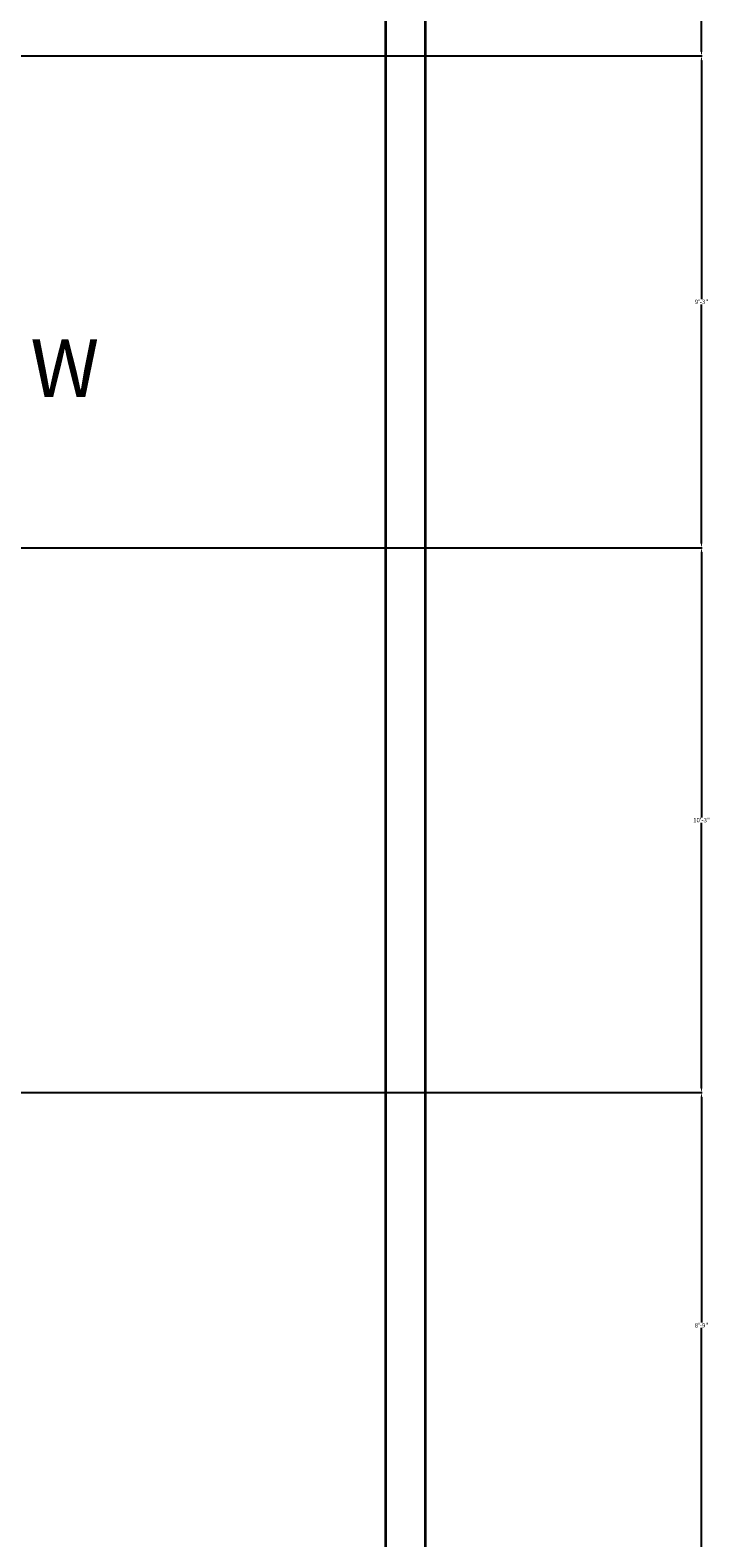
# Model space of a CAD drawing. Units: inches. Extents: x -364 to 705, y -52 to 1250.
# Tile 19 of 34: x 551 to 705, y 308 to 648. Entities that reach past the tile are written whole.
import ezdxf

# ---------------------------------------------------------------- set-up
doc = ezdxf.new("R2010")
doc.units = ezdxf.units.IN
doc.header["$MEASUREMENT"] = 0
for name, color, linetype, lineweight in [('A-ANNO-DIMS', 4, 'Continuous', 18), ('A-ANNO-IDEN', 1, 'Continuous', 18), ('C-WALL', 41, 'Continuous', 35)]:
    doc.layers.add(name, color=color, linetype=linetype, lineweight=lineweight)
doc.styles.get("Standard").update_dxf_attribs({"font": 'arial.ttf'})
doc.dimstyles.get("Standard").update_dxf_attribs({"dimtxt": 1, "dimasz": 1, "dimexe": 0.18, "dimexo": 0.0625, "dimgap": 0.09, "dimtad": 0, "dimtih": 1, "dimtoh": 1, "dimdec": 0, "dimzin": 0, "dimdsep": 46, "dimlunit": 3, "dimtxsty": 'Standard', "dimcen": 0.09, "dimadec": 0, "dimazin": 0, "dimtfac": 1, "dimtdec": 0, "dimtofl": 0, "dimtmove": 0, "dimatfit": 3, "dimfxl": 1, "dimtolj": 1, "dimtzin": 0, "dimarcsym": 0})

# ---------------------------------------------------------------- blocks, each defined once
blk = doc.blocks.new('*D79')
at = {"layer": 'A-ANNO-DIMS', "color": 0, "lineweight": -2, "transparency": 16777216}
for p, q in [((538.64, 408.11), (703.01, 408.11)), ((702.83, 407.11), (702.83, 356.22)), ((702.83, 304.11), (702.83, 355.01)), ((538.64, 303.11), (703.01, 303.11))]:
    blk.add_line(p, q, dxfattribs=at)
at = {"layer": 'A-ANNO-DIMS', "color": 0, "transparency": 16777216}
for points in [[(702.66, 407.11), (703, 407.11), (702.83, 408.11)], [(702.66, 304.11), (703, 304.11), (702.83, 303.11)]]:
    blk.add_solid(points, dxfattribs=at)
at = {"layer": 'Defpoints', "color": 0, "transparency": 16777216}
for p in [(538.58, 408.11), (702.83, 408.11), (538.58, 303.11)]:
    blk.add_point(p, dxfattribs=at)
at = {"layer": 'A-ANNO-DIMS', "color": 0, "transparency": 16777216, "insert": (702.83, 355.61), "char_height": 1, "attachment_point": 5}
blk.add_mtext('\\A1;8\'-9"', dxfattribs=at)
blk = doc.blocks.new('*D80')
at = {"layer": 'A-ANNO-DIMS', "color": 0, "lineweight": -2, "transparency": 16777216}
for p, q in [((538.64, 531.11), (703.01, 531.11)), ((702.83, 530.11), (702.83, 470.22)), ((702.83, 409.11), (702.83, 469.01)), ((538.64, 408.11), (703.01, 408.11))]:
    blk.add_line(p, q, dxfattribs=at)
at = {"layer": 'A-ANNO-DIMS', "color": 0, "transparency": 16777216}
for points in [[(702.66, 530.11), (703, 530.11), (702.83, 531.11)], [(702.66, 409.11), (703, 409.11), (702.83, 408.11)]]:
    blk.add_solid(points, dxfattribs=at)
at = {"layer": 'Defpoints', "color": 0, "transparency": 16777216}
for p in [(538.58, 531.11), (702.83, 531.11), (538.58, 408.11)]:
    blk.add_point(p, dxfattribs=at)
at = {"layer": 'A-ANNO-DIMS', "color": 0, "transparency": 16777216, "insert": (702.83, 469.61), "char_height": 1, "attachment_point": 5}
blk.add_mtext('\\A1;10\'-3"', dxfattribs=at)
blk = doc.blocks.new('*D81')
at = {"layer": 'A-ANNO-DIMS', "color": 0, "lineweight": -2, "transparency": 16777216}
for p, q in [((538.64, 642.11), (703.01, 642.11)), ((702.83, 641.11), (702.83, 587.22)), ((702.83, 532.11), (702.83, 586.01)), ((538.64, 531.11), (703.01, 531.11))]:
    blk.add_line(p, q, dxfattribs=at)
at = {"layer": 'A-ANNO-DIMS', "color": 0, "transparency": 16777216}
for points in [[(702.66, 641.11), (703, 641.11), (702.83, 642.11)], [(702.66, 532.11), (703, 532.11), (702.83, 531.11)]]:
    blk.add_solid(points, dxfattribs=at)
at = {"layer": 'Defpoints', "color": 0, "transparency": 16777216}
for p in [(538.58, 642.11), (702.83, 642.11), (538.58, 531.11)]:
    blk.add_point(p, dxfattribs=at)
at = {"layer": 'A-ANNO-DIMS', "color": 0, "transparency": 16777216, "insert": (702.83, 586.61), "char_height": 1, "attachment_point": 5}
blk.add_mtext('\\A1;9\'-3"', dxfattribs=at)
blk = doc.blocks.new('*D82')
at = {"layer": 'A-ANNO-DIMS', "color": 0, "lineweight": -2, "transparency": 16777216}
for p, q in [((538.64, 753.11), (703.01, 753.11)), ((702.83, 752.11), (702.83, 698.22)), ((702.83, 643.11), (702.83, 697.01)), ((538.64, 642.11), (703.01, 642.11))]:
    blk.add_line(p, q, dxfattribs=at)
at = {"layer": 'A-ANNO-DIMS', "color": 0, "transparency": 16777216}
for points in [[(702.66, 752.11), (703, 752.11), (702.83, 753.11)], [(702.66, 643.11), (703, 643.11), (702.83, 642.11)]]:
    blk.add_solid(points, dxfattribs=at)
at = {"layer": 'Defpoints', "color": 0, "transparency": 16777216}
for p in [(538.58, 753.11), (702.83, 753.11), (538.58, 642.11)]:
    blk.add_point(p, dxfattribs=at)
at = {"layer": 'A-ANNO-DIMS', "color": 0, "transparency": 16777216, "insert": (702.83, 697.61), "char_height": 1, "attachment_point": 5}
blk.add_mtext('\\A1;9\'-3"', dxfattribs=at)

msp = doc.modelspace()

# ---------------------------------------------------------------- linework, layer by layer
at = {"layer": 'C-WALL'}
for p, q in [((640.58, 11.11), (640.58, 1079.11)), ((631.58, 11.11), (631.58, 1070.11))]:
    msp.add_line(p, q, dxfattribs=at)

# ---------------------------------------------------------------- texts
at = {"layer": 'A-ANNO-IDEN', "insert": (551.36, 578.16), "char_height": 13, "attachment_point": 1}
msp.add_mtext_dynamic_manual_height_columns('W', width=33.6923, gutter_width=1, heights=[0], dxfattribs=at)

# ---------------------------------------------------------------- dimensions: what is measured, and where the dimension line sits
at = {"layer": 'A-ANNO-DIMS'}
for base, p1, p2, picture, middle in [((702.83, 753.11), (538.58, 642.11), (538.58, 753.11), '*D82', (702.83, 697.61)), ((702.83, 642.11), (538.58, 531.11), (538.58, 642.11), '*D81', (702.83, 586.61)), ((702.83, 531.11), (538.58, 408.11), (538.58, 531.11), '*D80', (702.83, 469.61)), ((702.83, 408.11), (538.58, 303.11), (538.58, 408.11), '*D79', (702.83, 355.61))]:
    dim = msp.add_linear_dim(base=base, p1=p1, p2=p2, angle=90, dimstyle='Standard', override={"dimdec": 1, "dimlfac": 1, "dimrnd": 0, "dimzin": 1, "dimdsep": 46, "dimlunit": 4, "dimfrac": 2}, dxfattribs=at)
    dim.commit()
    dim.dimension.update_dxf_attribs({"geometry": picture, "text_midpoint": middle})

doc.saveas('drawing.dxf')
